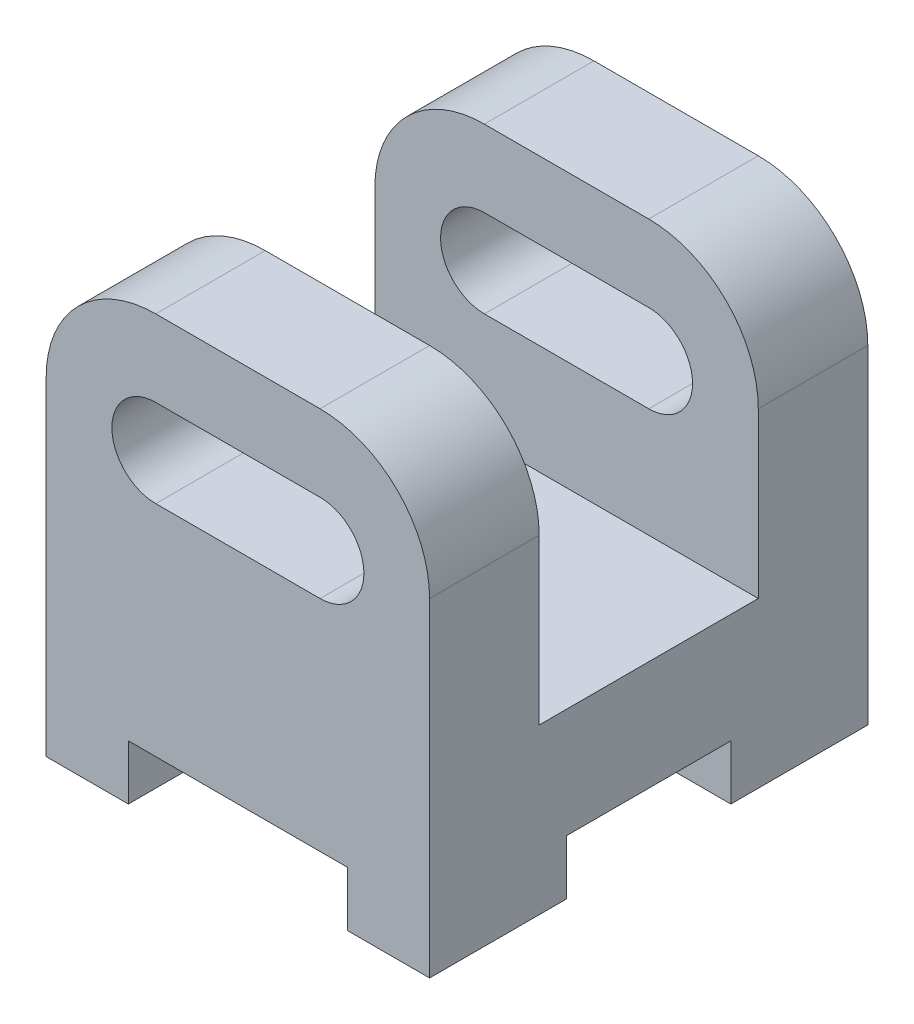
ISO-10303-21;
HEADER;
FILE_DESCRIPTION(('STEP AP214'),'2;1');
FILE_NAME('part.step','',(''),(''),'','','');
FILE_SCHEMA(('AUTOMOTIVE_DESIGN { 1 0 10303 214 1 1 1 1 }'));
ENDSEC;
DATA;
#1=APPLICATION_CONTEXT('core data for automotive mechanical design processes');
#2=APPLICATION_PROTOCOL_DEFINITION('international standard','automotive_design',2000,#1);
#3=PRODUCT_CONTEXT('',#1,'mechanical');
#4=PRODUCT('Part','Part','',(#3));
#5=PRODUCT_RELATED_PRODUCT_CATEGORY('part','',(#4));
#6=PRODUCT_DEFINITION_FORMATION('','',#4);
#7=PRODUCT_DEFINITION_CONTEXT('part definition',#1,'design');
#8=PRODUCT_DEFINITION('design','',#6,#7);
#9=PRODUCT_DEFINITION_SHAPE('','',#8);
#10=(LENGTH_UNIT() NAMED_UNIT(*) SI_UNIT(.MILLI.,.METRE.));
#11=(NAMED_UNIT(*) PLANE_ANGLE_UNIT() SI_UNIT($,.RADIAN.));
#12=(NAMED_UNIT(*) SI_UNIT($,.STERADIAN.) SOLID_ANGLE_UNIT());
#13=UNCERTAINTY_MEASURE_WITH_UNIT(LENGTH_MEASURE(1.E-05),#10,'distance_accuracy_value','');
#14=(GEOMETRIC_REPRESENTATION_CONTEXT(3) GLOBAL_UNCERTAINTY_ASSIGNED_CONTEXT((#13)) GLOBAL_UNIT_ASSIGNED_CONTEXT((#10,
#11,#12)) REPRESENTATION_CONTEXT('',''));
#15=CARTESIAN_POINT('',(0.,0.,0.));
#16=DIRECTION('',(0.,0.,1.));
#17=DIRECTION('',(1.,0.,0.));
#18=AXIS2_PLACEMENT_3D('',#15,#16,#17);
#19=CARTESIAN_POINT('',(35.,-40.,40.));
#20=DIRECTION('',(0.,1.,0.));
#21=DIRECTION('',(0.,0.,1.));
#22=AXIS2_PLACEMENT_3D('',#19,#20,#21);
#23=PLANE('',#22);
#24=DIRECTION('',(1.,0.,0.));
#25=VECTOR('',#24,1.);
#26=CARTESIAN_POINT('',(-35.,-40.,15.));
#27=LINE('',#26,#25);
#28=CARTESIAN_POINT('',(-35.,-40.,15.));
#29=VERTEX_POINT('',#28);
#30=CARTESIAN_POINT('',(-20.,-40.,15.));
#31=VERTEX_POINT('',#30);
#32=EDGE_CURVE('E367',#29,#31,#27,.T.);
#33=ORIENTED_EDGE('',*,*,#32,.T.);
#34=DIRECTION('',(0.,0.,1.));
#35=VECTOR('',#34,1.);
#36=CARTESIAN_POINT('',(-20.,-40.,-40.));
#37=LINE('',#36,#35);
#38=CARTESIAN_POINT('',(-20.,-40.,40.));
#39=VERTEX_POINT('',#38);
#40=EDGE_CURVE('E323',#31,#39,#37,.T.);
#41=ORIENTED_EDGE('',*,*,#40,.T.);
#42=DIRECTION('',(-1.,0.,0.));
#43=VECTOR('',#42,1.);
#44=CARTESIAN_POINT('',(35.,-40.,40.));
#45=LINE('',#44,#43);
#46=CARTESIAN_POINT('',(-35.,-40.,40.));
#47=VERTEX_POINT('',#46);
#48=EDGE_CURVE('E428',#39,#47,#45,.T.);
#49=ORIENTED_EDGE('',*,*,#48,.T.);
#50=DIRECTION('',(0.,0.,-1.));
#51=VECTOR('',#50,1.);
#52=CARTESIAN_POINT('',(-35.,-40.,40.));
#53=LINE('',#52,#51);
#54=EDGE_CURVE('E413',#47,#29,#53,.T.);
#55=ORIENTED_EDGE('',*,*,#54,.T.);
#56=EDGE_LOOP('',(#33,#41,#49,#55));
#57=FACE_BOUND('',#56,.T.);
#58=ADVANCED_FACE('F39',(#57),#23,.F.);
#59=DIRECTION('',(-1.,0.,0.));
#60=VECTOR('',#59,1.);
#61=CARTESIAN_POINT('',(35.,-40.,-40.));
#62=LINE('',#61,#60);
#63=CARTESIAN_POINT('',(-20.,-40.,-40.));
#64=VERTEX_POINT('',#63);
#65=CARTESIAN_POINT('',(-35.,-40.,-40.));
#66=VERTEX_POINT('',#65);
#67=EDGE_CURVE('E417',#64,#66,#62,.T.);
#68=ORIENTED_EDGE('',*,*,#67,.F.);
#69=CARTESIAN_POINT('',(-20.,-40.,-15.));
#70=VERTEX_POINT('',#69);
#71=EDGE_CURVE('E343',#64,#70,#37,.T.);
#72=ORIENTED_EDGE('',*,*,#71,.T.);
#73=DIRECTION('',(1.,0.,0.));
#74=VECTOR('',#73,1.);
#75=CARTESIAN_POINT('',(-35.,-40.,-15.));
#76=LINE('',#75,#74);
#77=CARTESIAN_POINT('',(-35.,-40.,-15.));
#78=VERTEX_POINT('',#77);
#79=EDGE_CURVE('E372',#78,#70,#76,.T.);
#80=ORIENTED_EDGE('',*,*,#79,.F.);
#81=EDGE_CURVE('E425',#78,#66,#53,.T.);
#82=ORIENTED_EDGE('',*,*,#81,.T.);
#83=EDGE_LOOP('',(#68,#72,#80,#82));
#84=FACE_BOUND('',#83,.T.);
#85=ADVANCED_FACE('F570',(#84),#23,.F.);
#86=CARTESIAN_POINT('',(-35.,-40.,-15.));
#87=DIRECTION('',(0.,0.,-1.));
#88=DIRECTION('',(-1.,0.,0.));
#89=AXIS2_PLACEMENT_3D('',#86,#87,#88);
#90=PLANE('',#89);
#91=ORIENTED_EDGE('',*,*,#79,.T.);
#92=DIRECTION('',(0.,1.,0.));
#93=VECTOR('',#92,1.);
#94=CARTESIAN_POINT('',(-20.,-40.,-15.));
#95=LINE('',#94,#93);
#96=CARTESIAN_POINT('',(-20.,-30.,-15.));
#97=VERTEX_POINT('',#96);
#98=EDGE_CURVE('E347',#70,#97,#95,.T.);
#99=ORIENTED_EDGE('',*,*,#98,.T.);
#100=DIRECTION('',(1.,0.,0.));
#101=VECTOR('',#100,1.);
#102=CARTESIAN_POINT('',(-35.,-30.,-15.));
#103=LINE('',#102,#101);
#104=CARTESIAN_POINT('',(-35.,-30.,-15.));
#105=VERTEX_POINT('',#104);
#106=EDGE_CURVE('E378',#105,#97,#103,.T.);
#107=ORIENTED_EDGE('',*,*,#106,.F.);
#108=DIRECTION('',(0.,1.,0.));
#109=VECTOR('',#108,1.);
#110=CARTESIAN_POINT('',(-35.,-40.,-15.));
#111=LINE('',#110,#109);
#112=EDGE_CURVE('E355',#78,#105,#111,.T.);
#113=ORIENTED_EDGE('',*,*,#112,.F.);
#114=EDGE_LOOP('',(#91,#99,#107,#113));
#115=FACE_BOUND('',#114,.T.);
#116=ADVANCED_FACE('F572',(#115),#90,.F.);
#117=CARTESIAN_POINT('',(-35.,-40.,15.));
#118=DIRECTION('',(0.,0.,-1.));
#119=DIRECTION('',(-1.,0.,0.));
#120=AXIS2_PLACEMENT_3D('',#117,#118,#119);
#121=PLANE('',#120);
#122=DIRECTION('',(0.,1.,0.));
#123=VECTOR('',#122,1.);
#124=CARTESIAN_POINT('',(-20.,-40.,15.));
#125=LINE('',#124,#123);
#126=CARTESIAN_POINT('',(-20.,-30.,15.));
#127=VERTEX_POINT('',#126);
#128=EDGE_CURVE('E439',#31,#127,#125,.T.);
#129=ORIENTED_EDGE('',*,*,#128,.F.);
#130=ORIENTED_EDGE('',*,*,#32,.F.);
#131=DIRECTION('',(0.,1.,0.));
#132=VECTOR('',#131,1.);
#133=CARTESIAN_POINT('',(-35.,-40.,15.));
#134=LINE('',#133,#132);
#135=CARTESIAN_POINT('',(-35.,-30.,15.));
#136=VERTEX_POINT('',#135);
#137=EDGE_CURVE('E358',#29,#136,#134,.T.);
#138=ORIENTED_EDGE('',*,*,#137,.T.);
#139=DIRECTION('',(1.,0.,0.));
#140=VECTOR('',#139,1.);
#141=CARTESIAN_POINT('',(-35.,-30.,15.));
#142=LINE('',#141,#140);
#143=EDGE_CURVE('E368',#136,#127,#142,.T.);
#144=ORIENTED_EDGE('',*,*,#143,.T.);
#145=EDGE_LOOP('',(#129,#130,#138,#144));
#146=FACE_BOUND('',#145,.T.);
#147=ADVANCED_FACE('F590',(#146),#121,.T.);
#148=CARTESIAN_POINT('',(35.,-40.,40.));
#149=VERTEX_POINT('',#148);
#150=CARTESIAN_POINT('',(20.,-40.,40.));
#151=VERTEX_POINT('',#150);
#152=EDGE_CURVE('E427',#149,#151,#45,.T.);
#153=ORIENTED_EDGE('',*,*,#152,.T.);
#154=DIRECTION('',(0.,0.,1.));
#155=VECTOR('',#154,1.);
#156=CARTESIAN_POINT('',(20.,-40.,-40.));
#157=LINE('',#156,#155);
#158=CARTESIAN_POINT('',(20.,-40.,15.));
#159=VERTEX_POINT('',#158);
#160=EDGE_CURVE('E339',#159,#151,#157,.T.);
#161=ORIENTED_EDGE('',*,*,#160,.F.);
#162=CARTESIAN_POINT('',(35.,-40.,15.));
#163=VERTEX_POINT('',#162);
#164=EDGE_CURVE('E369',#159,#163,#27,.T.);
#165=ORIENTED_EDGE('',*,*,#164,.T.);
#166=DIRECTION('',(0.,0.,-1.));
#167=VECTOR('',#166,1.);
#168=CARTESIAN_POINT('',(35.,-40.,40.));
#169=LINE('',#168,#167);
#170=EDGE_CURVE('E415',#149,#163,#169,.T.);
#171=ORIENTED_EDGE('',*,*,#170,.F.);
#172=EDGE_LOOP('',(#153,#161,#165,#171));
#173=FACE_BOUND('',#172,.T.);
#174=ADVANCED_FACE('F493',(#173),#23,.F.);
#175=CARTESIAN_POINT('',(35.,40.,40.));
#176=DIRECTION('',(0.,-1.,0.));
#177=DIRECTION('',(0.,0.,-1.));
#178=AXIS2_PLACEMENT_3D('',#175,#176,#177);
#179=PLANE('',#178);
#180=DIRECTION('',(-1.,0.,0.));
#181=VECTOR('',#180,1.);
#182=CARTESIAN_POINT('',(35.,40.,-40.));
#183=LINE('',#182,#181);
#184=CARTESIAN_POINT('',(15.,40.,-40.));
#185=VERTEX_POINT('',#184);
#186=CARTESIAN_POINT('',(-15.,40.,-40.));
#187=VERTEX_POINT('',#186);
#188=EDGE_CURVE('E434',#185,#187,#183,.T.);
#189=ORIENTED_EDGE('',*,*,#188,.T.);
#190=DIRECTION('',(0.,0.,1.));
#191=VECTOR('',#190,1.);
#192=CARTESIAN_POINT('',(-15.,40.,40.));
#193=LINE('',#192,#191);
#194=CARTESIAN_POINT('',(-15.,40.,-20.));
#195=VERTEX_POINT('',#194);
#196=EDGE_CURVE('E467',#187,#195,#193,.T.);
#197=ORIENTED_EDGE('',*,*,#196,.T.);
#198=DIRECTION('',(1.,0.,0.));
#199=VECTOR('',#198,1.);
#200=CARTESIAN_POINT('',(-35.,40.,-20.));
#201=LINE('',#200,#199);
#202=CARTESIAN_POINT('',(15.,40.,-20.));
#203=VERTEX_POINT('',#202);
#204=EDGE_CURVE('E401',#195,#203,#201,.T.);
#205=ORIENTED_EDGE('',*,*,#204,.T.);
#206=DIRECTION('',(0.,0.,1.));
#207=VECTOR('',#206,1.);
#208=CARTESIAN_POINT('',(15.,40.,-40.));
#209=LINE('',#208,#207);
#210=EDGE_CURVE('E468',#203,#185,#209,.F.);
#211=ORIENTED_EDGE('',*,*,#210,.T.);
#212=EDGE_LOOP('',(#189,#197,#205,#211));
#213=FACE_BOUND('',#212,.T.);
#214=ADVANCED_FACE('F516',(#213),#179,.F.);
#215=CARTESIAN_POINT('',(35.,40.,-40.));
#216=DIRECTION('',(0.,0.,1.));
#217=DIRECTION('',(0.,-1.,0.));
#218=AXIS2_PLACEMENT_3D('',#215,#216,#217);
#219=PLANE('',#218);
#220=DIRECTION('',(-1.,0.,0.));
#221=VECTOR('',#220,1.);
#222=CARTESIAN_POINT('',(-15.,26.,-40.));
#223=LINE('',#222,#221);
#224=CARTESIAN_POINT('',(15.,26.,-40.));
#225=VERTEX_POINT('',#224);
#226=CARTESIAN_POINT('',(-15.,26.,-40.));
#227=VERTEX_POINT('',#226);
#228=EDGE_CURVE('E277',#225,#227,#223,.T.);
#229=ORIENTED_EDGE('',*,*,#228,.T.);
#230=CARTESIAN_POINT('',(-15.,18.,-40.));
#231=DIRECTION('',(0.,0.,1.));
#232=DIRECTION('',(1.,0.,0.));
#233=AXIS2_PLACEMENT_3D('',#230,#231,#232);
#234=CIRCLE('',#233,8.);
#235=CARTESIAN_POINT('',(-15.,9.99999999999999,-40.));
#236=VERTEX_POINT('',#235);
#237=EDGE_CURVE('E254',#227,#236,#234,.T.);
#238=ORIENTED_EDGE('',*,*,#237,.T.);
#239=DIRECTION('',(1.,0.,0.));
#240=VECTOR('',#239,1.);
#241=CARTESIAN_POINT('',(-15.,9.99999999999999,-40.));
#242=LINE('',#241,#240);
#243=CARTESIAN_POINT('',(15.,9.99999999999999,-40.));
#244=VERTEX_POINT('',#243);
#245=EDGE_CURVE('E266',#236,#244,#242,.T.);
#246=ORIENTED_EDGE('',*,*,#245,.T.);
#247=CARTESIAN_POINT('',(15.,18.,-40.));
#248=DIRECTION('',(0.,0.,1.));
#249=DIRECTION('',(1.,0.,0.));
#250=AXIS2_PLACEMENT_3D('',#247,#248,#249);
#251=CIRCLE('',#250,8.);
#252=EDGE_CURVE('E275',#244,#225,#251,.T.);
#253=ORIENTED_EDGE('',*,*,#252,.T.);
#254=EDGE_LOOP('',(#229,#238,#246,#253));
#255=FACE_BOUND('',#254,.T.);
#256=DIRECTION('',(0.,1.,0.));
#257=VECTOR('',#256,1.);
#258=CARTESIAN_POINT('',(-35.,40.,-40.));
#259=LINE('',#258,#257);
#260=CARTESIAN_POINT('',(-35.,20.,-40.));
#261=VERTEX_POINT('',#260);
#262=EDGE_CURVE('E400',#66,#261,#259,.T.);
#263=ORIENTED_EDGE('',*,*,#262,.T.);
#264=CARTESIAN_POINT('',(-15.,20.,-40.));
#265=DIRECTION('',(0.,0.,1.));
#266=DIRECTION('',(0.,-1.,0.));
#267=AXIS2_PLACEMENT_3D('',#264,#265,#266);
#268=CIRCLE('',#267,20.);
#269=EDGE_CURVE('E474',#261,#187,#268,.F.);
#270=ORIENTED_EDGE('',*,*,#269,.T.);
#271=ORIENTED_EDGE('',*,*,#188,.F.);
#272=CARTESIAN_POINT('',(15.,20.,-40.));
#273=DIRECTION('',(0.,0.,1.));
#274=DIRECTION('',(0.,-1.,0.));
#275=AXIS2_PLACEMENT_3D('',#272,#273,#274);
#276=CIRCLE('',#275,20.);
#277=CARTESIAN_POINT('',(35.,20.,-40.));
#278=VERTEX_POINT('',#277);
#279=EDGE_CURVE('E53',#185,#278,#276,.F.);
#280=ORIENTED_EDGE('',*,*,#279,.T.);
#281=DIRECTION('',(0.,1.,0.));
#282=VECTOR('',#281,1.);
#283=CARTESIAN_POINT('',(35.,40.,-40.));
#284=LINE('',#283,#282);
#285=CARTESIAN_POINT('',(35.,-40.,-40.));
#286=VERTEX_POINT('',#285);
#287=EDGE_CURVE('E406',#286,#278,#284,.T.);
#288=ORIENTED_EDGE('',*,*,#287,.F.);
#289=CARTESIAN_POINT('',(20.,-40.,-40.));
#290=VERTEX_POINT('',#289);
#291=EDGE_CURVE('E422',#286,#290,#62,.T.);
#292=ORIENTED_EDGE('',*,*,#291,.T.);
#293=DIRECTION('',(0.,1.,0.));
#294=VECTOR('',#293,1.);
#295=CARTESIAN_POINT('',(20.,-40.,-40.));
#296=LINE('',#295,#294);
#297=CARTESIAN_POINT('',(20.,-30.,-40.));
#298=VERTEX_POINT('',#297);
#299=EDGE_CURVE('E316',#290,#298,#296,.T.);
#300=ORIENTED_EDGE('',*,*,#299,.T.);
#301=DIRECTION('',(-1.,0.,0.));
#302=VECTOR('',#301,1.);
#303=CARTESIAN_POINT('',(-20.,-30.,-40.));
#304=LINE('',#303,#302);
#305=CARTESIAN_POINT('',(-20.,-30.,-40.));
#306=VERTEX_POINT('',#305);
#307=EDGE_CURVE('E319',#298,#306,#304,.T.);
#308=ORIENTED_EDGE('',*,*,#307,.T.);
#309=DIRECTION('',(0.,-1.,0.));
#310=VECTOR('',#309,1.);
#311=CARTESIAN_POINT('',(-20.,-40.,-40.));
#312=LINE('',#311,#310);
#313=EDGE_CURVE('E311',#306,#64,#312,.T.);
#314=ORIENTED_EDGE('',*,*,#313,.T.);
#315=ORIENTED_EDGE('',*,*,#67,.T.);
#316=EDGE_LOOP('',(#263,#270,#271,#280,#288,#292,#300,#308,#314,#315));
#317=FACE_BOUND('',#316,.T.);
#318=ADVANCED_FACE('F273',(#255,#317),#219,.F.);
#319=DIRECTION('',(1.,0.,0.));
#320=VECTOR('',#319,1.);
#321=CARTESIAN_POINT('',(-35.,40.,20.));
#322=LINE('',#321,#320);
#323=CARTESIAN_POINT('',(-15.,40.,20.));
#324=VERTEX_POINT('',#323);
#325=CARTESIAN_POINT('',(15.,40.,20.));
#326=VERTEX_POINT('',#325);
#327=EDGE_CURVE('E396',#324,#326,#322,.T.);
#328=ORIENTED_EDGE('',*,*,#327,.F.);
#329=DIRECTION('',(0.,0.,1.));
#330=VECTOR('',#329,1.);
#331=CARTESIAN_POINT('',(-15.,40.,40.));
#332=LINE('',#331,#330);
#333=CARTESIAN_POINT('',(-15.,40.,40.));
#334=VERTEX_POINT('',#333);
#335=EDGE_CURVE('E453',#324,#334,#332,.T.);
#336=ORIENTED_EDGE('',*,*,#335,.T.);
#337=DIRECTION('',(-1.,0.,0.));
#338=VECTOR('',#337,1.);
#339=CARTESIAN_POINT('',(35.,40.,40.));
#340=LINE('',#339,#338);
#341=CARTESIAN_POINT('',(15.,40.,40.));
#342=VERTEX_POINT('',#341);
#343=EDGE_CURVE('E435',#342,#334,#340,.T.);
#344=ORIENTED_EDGE('',*,*,#343,.F.);
#345=DIRECTION('',(0.,0.,1.));
#346=VECTOR('',#345,1.);
#347=CARTESIAN_POINT('',(15.,40.,20.));
#348=LINE('',#347,#346);
#349=EDGE_CURVE('E447',#342,#326,#348,.F.);
#350=ORIENTED_EDGE('',*,*,#349,.T.);
#351=EDGE_LOOP('',(#328,#336,#344,#350));
#352=FACE_BOUND('',#351,.T.);
#353=ADVANCED_FACE('F541',(#352),#179,.F.);
#354=CARTESIAN_POINT('',(35.,40.,40.));
#355=DIRECTION('',(0.,0.,-1.));
#356=DIRECTION('',(-1.,0.,0.));
#357=AXIS2_PLACEMENT_3D('',#354,#355,#356);
#358=PLANE('',#357);
#359=DIRECTION('',(1.,0.,0.));
#360=VECTOR('',#359,1.);
#361=CARTESIAN_POINT('',(-15.,9.99999999999999,40.));
#362=LINE('',#361,#360);
#363=CARTESIAN_POINT('',(-15.,9.99999999999999,40.));
#364=VERTEX_POINT('',#363);
#365=CARTESIAN_POINT('',(15.,9.99999999999999,40.));
#366=VERTEX_POINT('',#365);
#367=EDGE_CURVE('E289',#364,#366,#362,.T.);
#368=ORIENTED_EDGE('',*,*,#367,.F.);
#369=CARTESIAN_POINT('',(-15.,18.,40.));
#370=DIRECTION('',(0.,0.,1.));
#371=DIRECTION('',(1.,0.,0.));
#372=AXIS2_PLACEMENT_3D('',#369,#370,#371);
#373=CIRCLE('',#372,8.);
#374=CARTESIAN_POINT('',(-15.,26.,40.));
#375=VERTEX_POINT('',#374);
#376=EDGE_CURVE('E284',#375,#364,#373,.T.);
#377=ORIENTED_EDGE('',*,*,#376,.F.);
#378=DIRECTION('',(-1.,0.,0.));
#379=VECTOR('',#378,1.);
#380=CARTESIAN_POINT('',(-15.,26.,40.));
#381=LINE('',#380,#379);
#382=CARTESIAN_POINT('',(15.,26.,40.));
#383=VERTEX_POINT('',#382);
#384=EDGE_CURVE('E280',#383,#375,#381,.T.);
#385=ORIENTED_EDGE('',*,*,#384,.F.);
#386=CARTESIAN_POINT('',(15.,18.,40.));
#387=DIRECTION('',(0.,0.,1.));
#388=DIRECTION('',(1.,0.,0.));
#389=AXIS2_PLACEMENT_3D('',#386,#387,#388);
#390=CIRCLE('',#389,8.);
#391=EDGE_CURVE('E278',#366,#383,#390,.T.);
#392=ORIENTED_EDGE('',*,*,#391,.F.);
#393=EDGE_LOOP('',(#368,#377,#385,#392));
#394=FACE_BOUND('',#393,.T.);
#395=ORIENTED_EDGE('',*,*,#343,.T.);
#396=CARTESIAN_POINT('',(-15.,20.,40.));
#397=DIRECTION('',(0.,0.,-1.));
#398=DIRECTION('',(-1.,0.,0.));
#399=AXIS2_PLACEMENT_3D('',#396,#397,#398);
#400=CIRCLE('',#399,20.);
#401=CARTESIAN_POINT('',(-35.,20.,40.));
#402=VERTEX_POINT('',#401);
#403=EDGE_CURVE('E457',#334,#402,#400,.F.);
#404=ORIENTED_EDGE('',*,*,#403,.T.);
#405=DIRECTION('',(0.,-1.,0.));
#406=VECTOR('',#405,1.);
#407=CARTESIAN_POINT('',(-35.,40.,40.));
#408=LINE('',#407,#406);
#409=EDGE_CURVE('E419',#402,#47,#408,.T.);
#410=ORIENTED_EDGE('',*,*,#409,.T.);
#411=ORIENTED_EDGE('',*,*,#48,.F.);
#412=DIRECTION('',(0.,-1.,0.));
#413=VECTOR('',#412,1.);
#414=CARTESIAN_POINT('',(-20.,-40.,40.));
#415=LINE('',#414,#413);
#416=CARTESIAN_POINT('',(-20.,-30.,40.));
#417=VERTEX_POINT('',#416);
#418=EDGE_CURVE('E315',#417,#39,#415,.T.);
#419=ORIENTED_EDGE('',*,*,#418,.F.);
#420=DIRECTION('',(-1.,0.,0.));
#421=VECTOR('',#420,1.);
#422=CARTESIAN_POINT('',(-20.,-30.,40.));
#423=LINE('',#422,#421);
#424=CARTESIAN_POINT('',(20.,-30.,40.));
#425=VERTEX_POINT('',#424);
#426=EDGE_CURVE('E320',#425,#417,#423,.T.);
#427=ORIENTED_EDGE('',*,*,#426,.F.);
#428=DIRECTION('',(0.,1.,0.));
#429=VECTOR('',#428,1.);
#430=CARTESIAN_POINT('',(20.,-40.,40.));
#431=LINE('',#430,#429);
#432=EDGE_CURVE('E324',#151,#425,#431,.T.);
#433=ORIENTED_EDGE('',*,*,#432,.F.);
#434=ORIENTED_EDGE('',*,*,#152,.F.);
#435=DIRECTION('',(0.,-1.,0.));
#436=VECTOR('',#435,1.);
#437=CARTESIAN_POINT('',(35.,40.,40.));
#438=LINE('',#437,#436);
#439=CARTESIAN_POINT('',(35.,20.,40.));
#440=VERTEX_POINT('',#439);
#441=EDGE_CURVE('E409',#440,#149,#438,.T.);
#442=ORIENTED_EDGE('',*,*,#441,.F.);
#443=CARTESIAN_POINT('',(15.,20.,40.));
#444=DIRECTION('',(0.,0.,-1.));
#445=DIRECTION('',(-1.,0.,0.));
#446=AXIS2_PLACEMENT_3D('',#443,#444,#445);
#447=CIRCLE('',#446,20.);
#448=EDGE_CURVE('E455',#440,#342,#447,.F.);
#449=ORIENTED_EDGE('',*,*,#448,.T.);
#450=EDGE_LOOP('',(#395,#404,#410,#411,#419,#427,#433,#434,#442,#449));
#451=FACE_BOUND('',#450,.T.);
#452=ADVANCED_FACE('F490',(#394,#451),#358,.F.);
#453=CARTESIAN_POINT('',(20.,-40.,-15.));
#454=VERTEX_POINT('',#453);
#455=CARTESIAN_POINT('',(35.,-40.,-15.));
#456=VERTEX_POINT('',#455);
#457=EDGE_CURVE('E373',#454,#456,#76,.T.);
#458=ORIENTED_EDGE('',*,*,#457,.F.);
#459=EDGE_CURVE('E336',#290,#454,#157,.T.);
#460=ORIENTED_EDGE('',*,*,#459,.F.);
#461=ORIENTED_EDGE('',*,*,#291,.F.);
#462=EDGE_CURVE('E412',#456,#286,#169,.T.);
#463=ORIENTED_EDGE('',*,*,#462,.F.);
#464=EDGE_LOOP('',(#458,#460,#461,#463));
#465=FACE_BOUND('',#464,.T.);
#466=ADVANCED_FACE('F511',(#465),#23,.F.);
#467=CARTESIAN_POINT('',(35.,0.,0.));
#468=DIRECTION('',(1.,0.,0.));
#469=DIRECTION('',(0.,0.,-1.));
#470=AXIS2_PLACEMENT_3D('',#467,#468,#469);
#471=PLANE('',#470);
#472=ORIENTED_EDGE('',*,*,#287,.T.);
#473=DIRECTION('',(0.,0.,1.));
#474=VECTOR('',#473,1.);
#475=CARTESIAN_POINT('',(35.,20.,-20.));
#476=LINE('',#475,#474);
#477=CARTESIAN_POINT('',(35.,20.,-20.));
#478=VERTEX_POINT('',#477);
#479=EDGE_CURVE('E11',#278,#478,#476,.T.);
#480=ORIENTED_EDGE('',*,*,#479,.T.);
#481=DIRECTION('',(0.,-1.,0.));
#482=VECTOR('',#481,1.);
#483=CARTESIAN_POINT('',(35.,40.,-20.));
#484=LINE('',#483,#482);
#485=CARTESIAN_POINT('',(35.,-10.,-20.));
#486=VERTEX_POINT('',#485);
#487=EDGE_CURVE('E391',#478,#486,#484,.T.);
#488=ORIENTED_EDGE('',*,*,#487,.T.);
#489=DIRECTION('',(0.,0.,-1.));
#490=VECTOR('',#489,1.);
#491=CARTESIAN_POINT('',(35.,-10.,20.));
#492=LINE('',#491,#490);
#493=CARTESIAN_POINT('',(35.,-10.,20.));
#494=VERTEX_POINT('',#493);
#495=EDGE_CURVE('E381',#494,#486,#492,.T.);
#496=ORIENTED_EDGE('',*,*,#495,.F.);
#497=DIRECTION('',(0.,-1.,0.));
#498=VECTOR('',#497,1.);
#499=CARTESIAN_POINT('',(35.,40.,20.));
#500=LINE('',#499,#498);
#501=CARTESIAN_POINT('',(35.,20.,20.));
#502=VERTEX_POINT('',#501);
#503=EDGE_CURVE('E387',#502,#494,#500,.T.);
#504=ORIENTED_EDGE('',*,*,#503,.F.);
#505=DIRECTION('',(0.,0.,1.));
#506=VECTOR('',#505,1.);
#507=CARTESIAN_POINT('',(35.,20.,40.));
#508=LINE('',#507,#506);
#509=EDGE_CURVE('E50',#502,#440,#508,.T.);
#510=ORIENTED_EDGE('',*,*,#509,.T.);
#511=ORIENTED_EDGE('',*,*,#441,.T.);
#512=ORIENTED_EDGE('',*,*,#170,.T.);
#513=DIRECTION('',(0.,1.,0.));
#514=VECTOR('',#513,1.);
#515=CARTESIAN_POINT('',(35.,-40.,15.));
#516=LINE('',#515,#514);
#517=CARTESIAN_POINT('',(35.,-30.,15.));
#518=VERTEX_POINT('',#517);
#519=EDGE_CURVE('E351',#163,#518,#516,.T.);
#520=ORIENTED_EDGE('',*,*,#519,.T.);
#521=DIRECTION('',(0.,0.,-1.));
#522=VECTOR('',#521,1.);
#523=CARTESIAN_POINT('',(35.,-30.,15.));
#524=LINE('',#523,#522);
#525=CARTESIAN_POINT('',(35.,-30.,-15.));
#526=VERTEX_POINT('',#525);
#527=EDGE_CURVE('E349',#518,#526,#524,.T.);
#528=ORIENTED_EDGE('',*,*,#527,.T.);
#529=DIRECTION('',(0.,1.,0.));
#530=VECTOR('',#529,1.);
#531=CARTESIAN_POINT('',(35.,-40.,-15.));
#532=LINE('',#531,#530);
#533=EDGE_CURVE('E363',#456,#526,#532,.T.);
#534=ORIENTED_EDGE('',*,*,#533,.F.);
#535=ORIENTED_EDGE('',*,*,#462,.T.);
#536=EDGE_LOOP('',(#472,#480,#488,#496,#504,#510,#511,#512,#520,#528,#534,#535));
#537=FACE_BOUND('',#536,.T.);
#538=ADVANCED_FACE('F481',(#537),#471,.T.);
#539=CARTESIAN_POINT('',(-35.,0.,0.));
#540=DIRECTION('',(1.,0.,0.));
#541=DIRECTION('',(0.,0.,-1.));
#542=AXIS2_PLACEMENT_3D('',#539,#540,#541);
#543=PLANE('',#542);
#544=ORIENTED_EDGE('',*,*,#409,.F.);
#545=DIRECTION('',(0.,0.,1.));
#546=VECTOR('',#545,1.);
#547=CARTESIAN_POINT('',(-35.,20.,0.));
#548=LINE('',#547,#546);
#549=CARTESIAN_POINT('',(-35.,20.,20.));
#550=VERTEX_POINT('',#549);
#551=EDGE_CURVE('E458',#402,#550,#548,.F.);
#552=ORIENTED_EDGE('',*,*,#551,.T.);
#553=DIRECTION('',(0.,-1.,0.));
#554=VECTOR('',#553,1.);
#555=CARTESIAN_POINT('',(-35.,40.,20.));
#556=LINE('',#555,#554);
#557=CARTESIAN_POINT('',(-35.,-10.,20.));
#558=VERTEX_POINT('',#557);
#559=EDGE_CURVE('E389',#550,#558,#556,.T.);
#560=ORIENTED_EDGE('',*,*,#559,.T.);
#561=DIRECTION('',(0.,0.,-1.));
#562=VECTOR('',#561,1.);
#563=CARTESIAN_POINT('',(-35.,-10.,20.));
#564=LINE('',#563,#562);
#565=CARTESIAN_POINT('',(-35.,-10.,-20.));
#566=VERTEX_POINT('',#565);
#567=EDGE_CURVE('E385',#558,#566,#564,.T.);
#568=ORIENTED_EDGE('',*,*,#567,.T.);
#569=DIRECTION('',(0.,-1.,0.));
#570=VECTOR('',#569,1.);
#571=CARTESIAN_POINT('',(-35.,40.,-20.));
#572=LINE('',#571,#570);
#573=CARTESIAN_POINT('',(-35.,20.,-20.));
#574=VERTEX_POINT('',#573);
#575=EDGE_CURVE('E384',#574,#566,#572,.T.);
#576=ORIENTED_EDGE('',*,*,#575,.F.);
#577=DIRECTION('',(0.,0.,1.));
#578=VECTOR('',#577,1.);
#579=CARTESIAN_POINT('',(-35.,20.,0.));
#580=LINE('',#579,#578);
#581=EDGE_CURVE('E456',#574,#261,#580,.F.);
#582=ORIENTED_EDGE('',*,*,#581,.T.);
#583=ORIENTED_EDGE('',*,*,#262,.F.);
#584=ORIENTED_EDGE('',*,*,#81,.F.);
#585=ORIENTED_EDGE('',*,*,#112,.T.);
#586=DIRECTION('',(0.,0.,-1.));
#587=VECTOR('',#586,1.);
#588=CARTESIAN_POINT('',(-35.,-30.,15.));
#589=LINE('',#588,#587);
#590=EDGE_CURVE('E348',#136,#105,#589,.T.);
#591=ORIENTED_EDGE('',*,*,#590,.F.);
#592=ORIENTED_EDGE('',*,*,#137,.F.);
#593=ORIENTED_EDGE('',*,*,#54,.F.);
#594=EDGE_LOOP('',(#544,#552,#560,#568,#576,#582,#583,#584,#585,#591,#592,#593));
#595=FACE_BOUND('',#594,.T.);
#596=ADVANCED_FACE('F549',(#595),#543,.F.);
#597=CARTESIAN_POINT('',(-35.,-10.,20.));
#598=DIRECTION('',(0.,-1.,0.));
#599=DIRECTION('',(0.,0.,-1.));
#600=AXIS2_PLACEMENT_3D('',#597,#598,#599);
#601=PLANE('',#600);
#602=ORIENTED_EDGE('',*,*,#495,.T.);
#603=DIRECTION('',(1.,0.,0.));
#604=VECTOR('',#603,1.);
#605=CARTESIAN_POINT('',(-35.,-10.,-20.));
#606=LINE('',#605,#604);
#607=EDGE_CURVE('E388',#566,#486,#606,.T.);
#608=ORIENTED_EDGE('',*,*,#607,.F.);
#609=ORIENTED_EDGE('',*,*,#567,.F.);
#610=DIRECTION('',(1.,0.,0.));
#611=VECTOR('',#610,1.);
#612=CARTESIAN_POINT('',(-35.,-10.,20.));
#613=LINE('',#612,#611);
#614=EDGE_CURVE('E398',#558,#494,#613,.T.);
#615=ORIENTED_EDGE('',*,*,#614,.T.);
#616=EDGE_LOOP('',(#602,#608,#609,#615));
#617=FACE_BOUND('',#616,.T.);
#618=ADVANCED_FACE('F533',(#617),#601,.F.);
#619=CARTESIAN_POINT('',(-35.,40.,20.));
#620=DIRECTION('',(0.,0.,1.));
#621=DIRECTION('',(0.,-1.,0.));
#622=AXIS2_PLACEMENT_3D('',#619,#620,#621);
#623=PLANE('',#622);
#624=DIRECTION('',(-1.,0.,0.));
#625=VECTOR('',#624,1.);
#626=CARTESIAN_POINT('',(-35.,26.,20.));
#627=LINE('',#626,#625);
#628=CARTESIAN_POINT('',(15.,26.,20.));
#629=VERTEX_POINT('',#628);
#630=CARTESIAN_POINT('',(-15.,26.,20.));
#631=VERTEX_POINT('',#630);
#632=EDGE_CURVE('E308',#629,#631,#627,.T.);
#633=ORIENTED_EDGE('',*,*,#632,.T.);
#634=CARTESIAN_POINT('',(-15.,18.,20.));
#635=DIRECTION('',(0.,0.,1.));
#636=DIRECTION('',(0.,-1.,0.));
#637=AXIS2_PLACEMENT_3D('',#634,#635,#636);
#638=CIRCLE('',#637,8.);
#639=CARTESIAN_POINT('',(-15.,9.99999999999999,20.));
#640=VERTEX_POINT('',#639);
#641=EDGE_CURVE('E310',#631,#640,#638,.T.);
#642=ORIENTED_EDGE('',*,*,#641,.T.);
#643=DIRECTION('',(1.,0.,0.));
#644=VECTOR('',#643,1.);
#645=CARTESIAN_POINT('',(-35.,9.99999999999999,20.));
#646=LINE('',#645,#644);
#647=CARTESIAN_POINT('',(15.,9.99999999999999,20.));
#648=VERTEX_POINT('',#647);
#649=EDGE_CURVE('E294',#640,#648,#646,.T.);
#650=ORIENTED_EDGE('',*,*,#649,.T.);
#651=CARTESIAN_POINT('',(15.,18.,20.));
#652=DIRECTION('',(0.,0.,1.));
#653=DIRECTION('',(0.,-1.,0.));
#654=AXIS2_PLACEMENT_3D('',#651,#652,#653);
#655=CIRCLE('',#654,8.);
#656=EDGE_CURVE('E302',#648,#629,#655,.T.);
#657=ORIENTED_EDGE('',*,*,#656,.T.);
#658=EDGE_LOOP('',(#633,#642,#650,#657));
#659=FACE_BOUND('',#658,.T.);
#660=ORIENTED_EDGE('',*,*,#559,.F.);
#661=CARTESIAN_POINT('',(-15.,20.,20.));
#662=DIRECTION('',(0.,0.,1.));
#663=DIRECTION('',(0.,-1.,0.));
#664=AXIS2_PLACEMENT_3D('',#661,#662,#663);
#665=CIRCLE('',#664,20.);
#666=EDGE_CURVE('E462',#550,#324,#665,.F.);
#667=ORIENTED_EDGE('',*,*,#666,.T.);
#668=ORIENTED_EDGE('',*,*,#327,.T.);
#669=CARTESIAN_POINT('',(15.,20.,20.));
#670=DIRECTION('',(0.,0.,1.));
#671=DIRECTION('',(0.,-1.,0.));
#672=AXIS2_PLACEMENT_3D('',#669,#670,#671);
#673=CIRCLE('',#672,20.);
#674=EDGE_CURVE('E465',#326,#502,#673,.F.);
#675=ORIENTED_EDGE('',*,*,#674,.T.);
#676=ORIENTED_EDGE('',*,*,#503,.T.);
#677=ORIENTED_EDGE('',*,*,#614,.F.);
#678=EDGE_LOOP('',(#660,#667,#668,#675,#676,#677));
#679=FACE_BOUND('',#678,.T.);
#680=ADVANCED_FACE('F536',(#659,#679),#623,.F.);
#681=CARTESIAN_POINT('',(-35.,40.,-20.));
#682=DIRECTION('',(0.,0.,1.));
#683=DIRECTION('',(0.,-1.,0.));
#684=AXIS2_PLACEMENT_3D('',#681,#682,#683);
#685=PLANE('',#684);
#686=CARTESIAN_POINT('',(-15.,18.,-20.));
#687=DIRECTION('',(0.,0.,1.));
#688=DIRECTION('',(0.,-1.,0.));
#689=AXIS2_PLACEMENT_3D('',#686,#687,#688);
#690=CIRCLE('',#689,8.);
#691=CARTESIAN_POINT('',(-15.,26.,-20.));
#692=VERTEX_POINT('',#691);
#693=CARTESIAN_POINT('',(-15.,9.99999999999999,-20.));
#694=VERTEX_POINT('',#693);
#695=EDGE_CURVE('E256',#692,#694,#690,.T.);
#696=ORIENTED_EDGE('',*,*,#695,.F.);
#697=DIRECTION('',(-1.,0.,0.));
#698=VECTOR('',#697,1.);
#699=CARTESIAN_POINT('',(-35.,26.,-20.));
#700=LINE('',#699,#698);
#701=CARTESIAN_POINT('',(15.,26.,-20.));
#702=VERTEX_POINT('',#701);
#703=EDGE_CURVE('E448',#702,#692,#700,.T.);
#704=ORIENTED_EDGE('',*,*,#703,.F.);
#705=CARTESIAN_POINT('',(15.,18.,-20.));
#706=DIRECTION('',(0.,0.,1.));
#707=DIRECTION('',(0.,-1.,0.));
#708=AXIS2_PLACEMENT_3D('',#705,#706,#707);
#709=CIRCLE('',#708,8.);
#710=CARTESIAN_POINT('',(15.,9.99999999999999,-20.));
#711=VERTEX_POINT('',#710);
#712=EDGE_CURVE('E441',#711,#702,#709,.T.);
#713=ORIENTED_EDGE('',*,*,#712,.F.);
#714=DIRECTION('',(1.,0.,0.));
#715=VECTOR('',#714,1.);
#716=CARTESIAN_POINT('',(-35.,9.99999999999999,-20.));
#717=LINE('',#716,#715);
#718=EDGE_CURVE('E445',#694,#711,#717,.T.);
#719=ORIENTED_EDGE('',*,*,#718,.F.);
#720=EDGE_LOOP('',(#696,#704,#713,#719));
#721=FACE_BOUND('',#720,.T.);
#722=ORIENTED_EDGE('',*,*,#204,.F.);
#723=CARTESIAN_POINT('',(-15.,20.,-20.));
#724=DIRECTION('',(0.,0.,1.));
#725=DIRECTION('',(0.,-1.,0.));
#726=AXIS2_PLACEMENT_3D('',#723,#724,#725);
#727=CIRCLE('',#726,20.);
#728=EDGE_CURVE('E472',#195,#574,#727,.T.);
#729=ORIENTED_EDGE('',*,*,#728,.T.);
#730=ORIENTED_EDGE('',*,*,#575,.T.);
#731=ORIENTED_EDGE('',*,*,#607,.T.);
#732=ORIENTED_EDGE('',*,*,#487,.F.);
#733=CARTESIAN_POINT('',(15.,20.,-20.));
#734=DIRECTION('',(0.,0.,1.));
#735=DIRECTION('',(0.,-1.,0.));
#736=AXIS2_PLACEMENT_3D('',#733,#734,#735);
#737=CIRCLE('',#736,20.);
#738=EDGE_CURVE('E65',#478,#203,#737,.T.);
#739=ORIENTED_EDGE('',*,*,#738,.T.);
#740=EDGE_LOOP('',(#722,#729,#730,#731,#732,#739));
#741=FACE_BOUND('',#740,.T.);
#742=ADVANCED_FACE('F527',(#721,#741),#685,.T.);
#743=CARTESIAN_POINT('',(-35.,-30.,15.));
#744=DIRECTION('',(0.,-1.,0.));
#745=DIRECTION('',(0.,0.,-1.));
#746=AXIS2_PLACEMENT_3D('',#743,#744,#745);
#747=PLANE('',#746);
#748=CARTESIAN_POINT('',(20.,-30.,15.));
#749=VERTEX_POINT('',#748);
#750=EDGE_CURVE('E357',#749,#518,#142,.T.);
#751=ORIENTED_EDGE('',*,*,#750,.F.);
#752=DIRECTION('',(0.,0.,1.));
#753=VECTOR('',#752,1.);
#754=CARTESIAN_POINT('',(20.,-30.,-40.));
#755=LINE('',#754,#753);
#756=EDGE_CURVE('E340',#749,#425,#755,.T.);
#757=ORIENTED_EDGE('',*,*,#756,.T.);
#758=ORIENTED_EDGE('',*,*,#426,.T.);
#759=DIRECTION('',(0.,0.,1.));
#760=VECTOR('',#759,1.);
#761=CARTESIAN_POINT('',(-20.,-30.,-40.));
#762=LINE('',#761,#760);
#763=EDGE_CURVE('E334',#127,#417,#762,.T.);
#764=ORIENTED_EDGE('',*,*,#763,.F.);
#765=ORIENTED_EDGE('',*,*,#143,.F.);
#766=ORIENTED_EDGE('',*,*,#590,.T.);
#767=ORIENTED_EDGE('',*,*,#106,.T.);
#768=EDGE_CURVE('E329',#306,#97,#762,.T.);
#769=ORIENTED_EDGE('',*,*,#768,.F.);
#770=ORIENTED_EDGE('',*,*,#307,.F.);
#771=CARTESIAN_POINT('',(20.,-30.,-15.));
#772=VERTEX_POINT('',#771);
#773=EDGE_CURVE('E331',#298,#772,#755,.T.);
#774=ORIENTED_EDGE('',*,*,#773,.T.);
#775=EDGE_CURVE('E380',#772,#526,#103,.T.);
#776=ORIENTED_EDGE('',*,*,#775,.T.);
#777=ORIENTED_EDGE('',*,*,#527,.F.);
#778=EDGE_LOOP('',(#751,#757,#758,#764,#765,#766,#767,#769,#770,#774,#776,#777));
#779=FACE_BOUND('',#778,.T.);
#780=ADVANCED_FACE('F502',(#779),#747,.T.);
#781=ORIENTED_EDGE('',*,*,#775,.F.);
#782=DIRECTION('',(0.,-1.,0.));
#783=VECTOR('',#782,1.);
#784=CARTESIAN_POINT('',(20.,-40.,-15.));
#785=LINE('',#784,#783);
#786=EDGE_CURVE('E335',#772,#454,#785,.T.);
#787=ORIENTED_EDGE('',*,*,#786,.T.);
#788=ORIENTED_EDGE('',*,*,#457,.T.);
#789=ORIENTED_EDGE('',*,*,#533,.T.);
#790=EDGE_LOOP('',(#781,#787,#788,#789));
#791=FACE_BOUND('',#790,.T.);
#792=ADVANCED_FACE('F507',(#791),#90,.F.);
#793=DIRECTION('',(0.,-1.,0.));
#794=VECTOR('',#793,1.);
#795=CARTESIAN_POINT('',(20.,-40.,15.));
#796=LINE('',#795,#794);
#797=EDGE_CURVE('E437',#749,#159,#796,.T.);
#798=ORIENTED_EDGE('',*,*,#797,.F.);
#799=ORIENTED_EDGE('',*,*,#750,.T.);
#800=ORIENTED_EDGE('',*,*,#519,.F.);
#801=ORIENTED_EDGE('',*,*,#164,.F.);
#802=EDGE_LOOP('',(#798,#799,#800,#801));
#803=FACE_BOUND('',#802,.T.);
#804=ADVANCED_FACE('F503',(#803),#121,.T.);
#805=CARTESIAN_POINT('',(20.,-40.,-40.));
#806=DIRECTION('',(1.,0.,0.));
#807=DIRECTION('',(0.,0.,-1.));
#808=AXIS2_PLACEMENT_3D('',#805,#806,#807);
#809=PLANE('',#808);
#810=ORIENTED_EDGE('',*,*,#797,.T.);
#811=ORIENTED_EDGE('',*,*,#160,.T.);
#812=ORIENTED_EDGE('',*,*,#432,.T.);
#813=ORIENTED_EDGE('',*,*,#756,.F.);
#814=EDGE_LOOP('',(#810,#811,#812,#813));
#815=FACE_BOUND('',#814,.T.);
#816=ADVANCED_FACE('F602',(#815),#809,.F.);
#817=CARTESIAN_POINT('',(-20.,-40.,-40.));
#818=DIRECTION('',(-1.,0.,0.));
#819=DIRECTION('',(0.,0.,1.));
#820=AXIS2_PLACEMENT_3D('',#817,#818,#819);
#821=PLANE('',#820);
#822=ORIENTED_EDGE('',*,*,#128,.T.);
#823=ORIENTED_EDGE('',*,*,#763,.T.);
#824=ORIENTED_EDGE('',*,*,#418,.T.);
#825=ORIENTED_EDGE('',*,*,#40,.F.);
#826=EDGE_LOOP('',(#822,#823,#824,#825));
#827=FACE_BOUND('',#826,.T.);
#828=ADVANCED_FACE('F609',(#827),#821,.F.);
#829=ORIENTED_EDGE('',*,*,#71,.F.);
#830=ORIENTED_EDGE('',*,*,#313,.F.);
#831=ORIENTED_EDGE('',*,*,#768,.T.);
#832=ORIENTED_EDGE('',*,*,#98,.F.);
#833=EDGE_LOOP('',(#829,#830,#831,#832));
#834=FACE_BOUND('',#833,.T.);
#835=ADVANCED_FACE('F686',(#834),#821,.F.);
#836=ORIENTED_EDGE('',*,*,#773,.F.);
#837=ORIENTED_EDGE('',*,*,#299,.F.);
#838=ORIENTED_EDGE('',*,*,#459,.T.);
#839=ORIENTED_EDGE('',*,*,#786,.F.);
#840=EDGE_LOOP('',(#836,#837,#838,#839));
#841=FACE_BOUND('',#840,.T.);
#842=ADVANCED_FACE('F613',(#841),#809,.F.);
#843=CARTESIAN_POINT('',(-15.,9.99999999999999,-40.));
#844=DIRECTION('',(0.,-1.,0.));
#845=DIRECTION('',(0.,0.,-1.));
#846=AXIS2_PLACEMENT_3D('',#843,#844,#845);
#847=PLANE('',#846);
#848=ORIENTED_EDGE('',*,*,#718,.T.);
#849=DIRECTION('',(0.,0.,1.));
#850=VECTOR('',#849,1.);
#851=CARTESIAN_POINT('',(15.,9.99999999999999,-40.));
#852=LINE('',#851,#850);
#853=EDGE_CURVE('E267',#244,#711,#852,.T.);
#854=ORIENTED_EDGE('',*,*,#853,.F.);
#855=ORIENTED_EDGE('',*,*,#245,.F.);
#856=DIRECTION('',(0.,0.,1.));
#857=VECTOR('',#856,1.);
#858=CARTESIAN_POINT('',(-15.,9.99999999999999,-40.));
#859=LINE('',#858,#857);
#860=EDGE_CURVE('E246',#236,#694,#859,.T.);
#861=ORIENTED_EDGE('',*,*,#860,.T.);
#862=EDGE_LOOP('',(#848,#854,#855,#861));
#863=FACE_BOUND('',#862,.T.);
#864=ADVANCED_FACE('F270',(#863),#847,.F.);
#865=CARTESIAN_POINT('',(15.,18.,-40.));
#866=DIRECTION('',(0.,0.,1.));
#867=DIRECTION('',(1.,0.,0.));
#868=AXIS2_PLACEMENT_3D('',#865,#866,#867);
#869=CYLINDRICAL_SURFACE('',#868,8.);
#870=ORIENTED_EDGE('',*,*,#712,.T.);
#871=DIRECTION('',(0.,0.,1.));
#872=VECTOR('',#871,1.);
#873=CARTESIAN_POINT('',(15.,26.,-40.));
#874=LINE('',#873,#872);
#875=EDGE_CURVE('E298',#225,#702,#874,.T.);
#876=ORIENTED_EDGE('',*,*,#875,.F.);
#877=ORIENTED_EDGE('',*,*,#252,.F.);
#878=ORIENTED_EDGE('',*,*,#853,.T.);
#879=EDGE_LOOP('',(#870,#876,#877,#878));
#880=FACE_BOUND('',#879,.T.);
#881=ADVANCED_FACE('F715',(#880),#869,.F.);
#882=CARTESIAN_POINT('',(-15.,26.,-40.));
#883=DIRECTION('',(0.,1.,0.));
#884=DIRECTION('',(0.,0.,1.));
#885=AXIS2_PLACEMENT_3D('',#882,#883,#884);
#886=PLANE('',#885);
#887=ORIENTED_EDGE('',*,*,#703,.T.);
#888=DIRECTION('',(0.,0.,1.));
#889=VECTOR('',#888,1.);
#890=CARTESIAN_POINT('',(-15.,26.,-40.));
#891=LINE('',#890,#889);
#892=EDGE_CURVE('E295',#227,#692,#891,.T.);
#893=ORIENTED_EDGE('',*,*,#892,.F.);
#894=ORIENTED_EDGE('',*,*,#228,.F.);
#895=ORIENTED_EDGE('',*,*,#875,.T.);
#896=EDGE_LOOP('',(#887,#893,#894,#895));
#897=FACE_BOUND('',#896,.T.);
#898=ADVANCED_FACE('F716',(#897),#886,.F.);
#899=CARTESIAN_POINT('',(-15.,18.,-40.));
#900=DIRECTION('',(0.,0.,1.));
#901=DIRECTION('',(1.,0.,0.));
#902=AXIS2_PLACEMENT_3D('',#899,#900,#901);
#903=CYLINDRICAL_SURFACE('',#902,8.);
#904=ORIENTED_EDGE('',*,*,#695,.T.);
#905=ORIENTED_EDGE('',*,*,#860,.F.);
#906=ORIENTED_EDGE('',*,*,#237,.F.);
#907=ORIENTED_EDGE('',*,*,#892,.T.);
#908=EDGE_LOOP('',(#904,#905,#906,#907));
#909=FACE_BOUND('',#908,.T.);
#910=ADVANCED_FACE('F252',(#909),#903,.F.);
#911=EDGE_CURVE('E293',#631,#375,#891,.T.);
#912=ORIENTED_EDGE('',*,*,#911,.T.);
#913=ORIENTED_EDGE('',*,*,#376,.T.);
#914=EDGE_CURVE('E265',#640,#364,#859,.T.);
#915=ORIENTED_EDGE('',*,*,#914,.F.);
#916=ORIENTED_EDGE('',*,*,#641,.F.);
#917=EDGE_LOOP('',(#912,#913,#915,#916));
#918=FACE_BOUND('',#917,.T.);
#919=ADVANCED_FACE('F740',(#918),#903,.F.);
#920=EDGE_CURVE('E297',#629,#383,#874,.T.);
#921=ORIENTED_EDGE('',*,*,#920,.T.);
#922=ORIENTED_EDGE('',*,*,#384,.T.);
#923=ORIENTED_EDGE('',*,*,#911,.F.);
#924=ORIENTED_EDGE('',*,*,#632,.F.);
#925=EDGE_LOOP('',(#921,#922,#923,#924));
#926=FACE_BOUND('',#925,.T.);
#927=ADVANCED_FACE('F726',(#926),#886,.F.);
#928=EDGE_CURVE('E261',#648,#366,#852,.T.);
#929=ORIENTED_EDGE('',*,*,#928,.T.);
#930=ORIENTED_EDGE('',*,*,#391,.T.);
#931=ORIENTED_EDGE('',*,*,#920,.F.);
#932=ORIENTED_EDGE('',*,*,#656,.F.);
#933=EDGE_LOOP('',(#929,#930,#931,#932));
#934=FACE_BOUND('',#933,.T.);
#935=ADVANCED_FACE('F564',(#934),#869,.F.);
#936=ORIENTED_EDGE('',*,*,#914,.T.);
#937=ORIENTED_EDGE('',*,*,#367,.T.);
#938=ORIENTED_EDGE('',*,*,#928,.F.);
#939=ORIENTED_EDGE('',*,*,#649,.F.);
#940=EDGE_LOOP('',(#936,#937,#938,#939));
#941=FACE_BOUND('',#940,.T.);
#942=ADVANCED_FACE('F551',(#941),#847,.F.);
#943=CARTESIAN_POINT('',(-15.,20.,40.));
#944=DIRECTION('',(0.,0.,1.));
#945=DIRECTION('',(1.,0.,0.));
#946=AXIS2_PLACEMENT_3D('',#943,#944,#945);
#947=CYLINDRICAL_SURFACE('',#946,20.);
#948=ORIENTED_EDGE('',*,*,#666,.F.);
#949=ORIENTED_EDGE('',*,*,#551,.F.);
#950=ORIENTED_EDGE('',*,*,#403,.F.);
#951=ORIENTED_EDGE('',*,*,#335,.F.);
#952=EDGE_LOOP('',(#948,#949,#950,#951));
#953=FACE_BOUND('',#952,.T.);
#954=ADVANCED_FACE('F555',(#953),#947,.T.);
#955=CARTESIAN_POINT('',(-15.,20.,40.));
#956=DIRECTION('',(0.,0.,1.));
#957=DIRECTION('',(1.,0.,0.));
#958=AXIS2_PLACEMENT_3D('',#955,#956,#957);
#959=CYLINDRICAL_SURFACE('',#958,20.);
#960=ORIENTED_EDGE('',*,*,#269,.F.);
#961=ORIENTED_EDGE('',*,*,#581,.F.);
#962=ORIENTED_EDGE('',*,*,#728,.F.);
#963=ORIENTED_EDGE('',*,*,#196,.F.);
#964=EDGE_LOOP('',(#960,#961,#962,#963));
#965=FACE_BOUND('',#964,.T.);
#966=ADVANCED_FACE('F521',(#965),#959,.T.);
#967=CARTESIAN_POINT('',(15.,20.,0.));
#968=DIRECTION('',(0.,0.,-1.));
#969=DIRECTION('',(-1.,0.,0.));
#970=AXIS2_PLACEMENT_3D('',#967,#968,#969);
#971=CYLINDRICAL_SURFACE('',#970,20.);
#972=ORIENTED_EDGE('',*,*,#279,.F.);
#973=ORIENTED_EDGE('',*,*,#210,.F.);
#974=ORIENTED_EDGE('',*,*,#738,.F.);
#975=ORIENTED_EDGE('',*,*,#479,.F.);
#976=EDGE_LOOP('',(#972,#973,#974,#975));
#977=FACE_BOUND('',#976,.T.);
#978=ADVANCED_FACE('F518',(#977),#971,.T.);
#979=CARTESIAN_POINT('',(15.,20.,0.));
#980=DIRECTION('',(0.,0.,-1.));
#981=DIRECTION('',(-1.,0.,0.));
#982=AXIS2_PLACEMENT_3D('',#979,#980,#981);
#983=CYLINDRICAL_SURFACE('',#982,20.);
#984=ORIENTED_EDGE('',*,*,#674,.F.);
#985=ORIENTED_EDGE('',*,*,#349,.F.);
#986=ORIENTED_EDGE('',*,*,#448,.F.);
#987=ORIENTED_EDGE('',*,*,#509,.F.);
#988=EDGE_LOOP('',(#984,#985,#986,#987));
#989=FACE_BOUND('',#988,.T.);
#990=ADVANCED_FACE('F41',(#989),#983,.T.);
#991=CLOSED_SHELL('',(#58,#85,#116,#147,#174,#214,#318,#353,#452,#466,#538,#596,#618,#680,#742,
#780,#792,#804,#816,#828,#835,#842,#864,#881,#898,#910,#919,#927,#935,#942,#954,#966,#978,#990));
#992=MANIFOLD_SOLID_BREP('B2',#991);
#993=ADVANCED_BREP_SHAPE_REPRESENTATION('',(#18,#992),#14);
#994=SHAPE_DEFINITION_REPRESENTATION(#9,#993);
ENDSEC;
END-ISO-10303-21;
